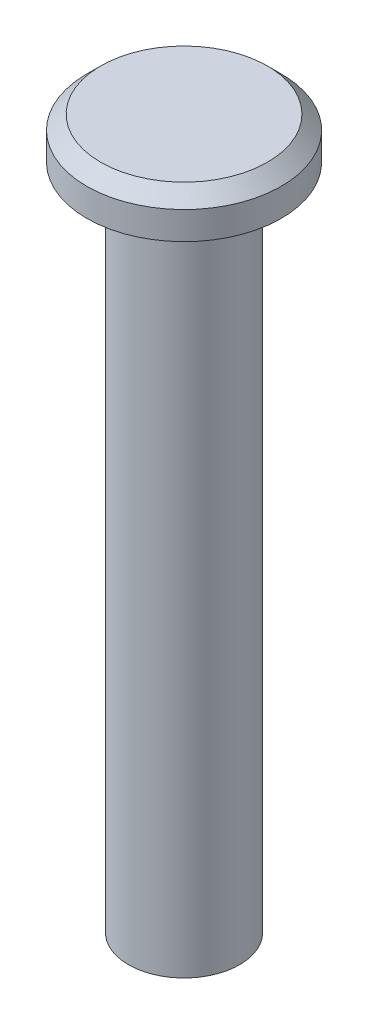
ISO-10303-21;
HEADER;
FILE_DESCRIPTION(('STEP AP214'),'2;1');
FILE_NAME('part.step','',(''),(''),'','','');
FILE_SCHEMA(('AUTOMOTIVE_DESIGN { 1 0 10303 214 1 1 1 1 }'));
ENDSEC;
DATA;
#1=APPLICATION_CONTEXT('core data for automotive mechanical design processes');
#2=APPLICATION_PROTOCOL_DEFINITION('international standard','automotive_design',2000,#1);
#3=PRODUCT_CONTEXT('',#1,'mechanical');
#4=PRODUCT('Part','Part','',(#3));
#5=PRODUCT_RELATED_PRODUCT_CATEGORY('part','',(#4));
#6=PRODUCT_DEFINITION_FORMATION('','',#4);
#7=PRODUCT_DEFINITION_CONTEXT('part definition',#1,'design');
#8=PRODUCT_DEFINITION('design','',#6,#7);
#9=PRODUCT_DEFINITION_SHAPE('','',#8);
#10=(LENGTH_UNIT() NAMED_UNIT(*) SI_UNIT(.MILLI.,.METRE.));
#11=(NAMED_UNIT(*) PLANE_ANGLE_UNIT() SI_UNIT($,.RADIAN.));
#12=(NAMED_UNIT(*) SI_UNIT($,.STERADIAN.) SOLID_ANGLE_UNIT());
#13=UNCERTAINTY_MEASURE_WITH_UNIT(LENGTH_MEASURE(1.E-05),#10,'distance_accuracy_value','');
#14=(GEOMETRIC_REPRESENTATION_CONTEXT(3) GLOBAL_UNCERTAINTY_ASSIGNED_CONTEXT((#13)) GLOBAL_UNIT_ASSIGNED_CONTEXT((#10,
#11,#12)) REPRESENTATION_CONTEXT('',''));
#15=CARTESIAN_POINT('',(0.,0.,0.));
#16=DIRECTION('',(0.,0.,1.));
#17=DIRECTION('',(1.,0.,0.));
#18=AXIS2_PLACEMENT_3D('',#15,#16,#17);
#19=CARTESIAN_POINT('',(0.,48.,0.));
#20=DIRECTION('',(0.,-1.,0.));
#21=DIRECTION('',(0.,0.,-1.));
#22=AXIS2_PLACEMENT_3D('',#19,#20,#21);
#23=CYLINDRICAL_SURFACE('',#22,4.);
#24=CARTESIAN_POINT('',(0.,48.,0.));
#25=DIRECTION('',(0.,1.,0.));
#26=DIRECTION('',(0.,0.,1.));
#27=AXIS2_PLACEMENT_3D('',#24,#25,#26);
#28=CIRCLE('',#27,4.);
#29=CARTESIAN_POINT('',(0.,48.,4.));
#30=VERTEX_POINT('',#29);
#31=EDGE_CURVE('E52',#30,#30,#28,.T.);
#32=ORIENTED_EDGE('',*,*,#31,.F.);
#33=EDGE_LOOP('',(#32));
#34=FACE_BOUND('',#33,.T.);
#35=CARTESIAN_POINT('',(0.,0.,0.));
#36=DIRECTION('',(0.,1.,0.));
#37=DIRECTION('',(0.,0.,1.));
#38=AXIS2_PLACEMENT_3D('',#35,#36,#37);
#39=CIRCLE('',#38,4.);
#40=CARTESIAN_POINT('',(0.,0.,4.));
#41=VERTEX_POINT('',#40);
#42=EDGE_CURVE('E60',#41,#41,#39,.T.);
#43=ORIENTED_EDGE('',*,*,#42,.T.);
#44=EDGE_LOOP('',(#43));
#45=FACE_BOUND('',#44,.T.);
#46=ADVANCED_FACE('F41',(#34,#45),#23,.T.);
#47=CARTESIAN_POINT('',(0.,0.,0.));
#48=DIRECTION('',(0.,1.,0.));
#49=DIRECTION('',(0.,0.,1.));
#50=AXIS2_PLACEMENT_3D('',#47,#48,#49);
#51=PLANE('',#50);
#52=ORIENTED_EDGE('',*,*,#42,.F.);
#53=EDGE_LOOP('',(#52));
#54=FACE_BOUND('',#53,.T.);
#55=ADVANCED_FACE('F83',(#54),#51,.F.);
#56=CARTESIAN_POINT('',(0.,51.,0.));
#57=DIRECTION('',(0.,-1.,0.));
#58=DIRECTION('',(0.,0.,-1.));
#59=AXIS2_PLACEMENT_3D('',#56,#57,#58);
#60=CYLINDRICAL_SURFACE('',#59,7.);
#61=CARTESIAN_POINT('',(0.,50.,0.));
#62=DIRECTION('',(0.,1.,0.));
#63=DIRECTION('',(0.,0.,1.));
#64=AXIS2_PLACEMENT_3D('',#61,#62,#63);
#65=CIRCLE('',#64,7.);
#66=CARTESIAN_POINT('',(0.,50.,7.));
#67=VERTEX_POINT('',#66);
#68=EDGE_CURVE('E10',#67,#67,#65,.F.);
#69=ORIENTED_EDGE('',*,*,#68,.T.);
#70=EDGE_LOOP('',(#69));
#71=FACE_BOUND('',#70,.T.);
#72=CARTESIAN_POINT('',(0.,48.,0.));
#73=DIRECTION('',(0.,1.,0.));
#74=DIRECTION('',(0.,0.,1.));
#75=AXIS2_PLACEMENT_3D('',#72,#73,#74);
#76=CIRCLE('',#75,7.);
#77=CARTESIAN_POINT('',(0.,48.,7.));
#78=VERTEX_POINT('',#77);
#79=EDGE_CURVE('E61',#78,#78,#76,.T.);
#80=ORIENTED_EDGE('',*,*,#79,.T.);
#81=EDGE_LOOP('',(#80));
#82=FACE_BOUND('',#81,.T.);
#83=ADVANCED_FACE('F66',(#71,#82),#60,.T.);
#84=CARTESIAN_POINT('',(0.,51.,0.));
#85=DIRECTION('',(0.,1.,0.));
#86=DIRECTION('',(0.,0.,1.));
#87=AXIS2_PLACEMENT_3D('',#84,#85,#86);
#88=PLANE('',#87);
#89=CARTESIAN_POINT('',(0.,51.,0.));
#90=DIRECTION('',(0.,1.,0.));
#91=DIRECTION('',(0.,0.,1.));
#92=AXIS2_PLACEMENT_3D('',#89,#90,#91);
#93=CIRCLE('',#92,6.);
#94=CARTESIAN_POINT('',(0.,51.,6.));
#95=VERTEX_POINT('',#94);
#96=EDGE_CURVE('E47',#95,#95,#93,.T.);
#97=ORIENTED_EDGE('',*,*,#96,.T.);
#98=EDGE_LOOP('',(#97));
#99=FACE_BOUND('',#98,.T.);
#100=ADVANCED_FACE('F69',(#99),#88,.T.);
#101=CARTESIAN_POINT('',(0.,48.,0.));
#102=DIRECTION('',(0.,1.,0.));
#103=DIRECTION('',(0.,0.,1.));
#104=AXIS2_PLACEMENT_3D('',#101,#102,#103);
#105=PLANE('',#104);
#106=ORIENTED_EDGE('',*,*,#31,.T.);
#107=EDGE_LOOP('',(#106));
#108=FACE_BOUND('',#107,.T.);
#109=ORIENTED_EDGE('',*,*,#79,.F.);
#110=EDGE_LOOP('',(#109));
#111=FACE_BOUND('',#110,.T.);
#112=ADVANCED_FACE('F68',(#108,#111),#105,.F.);
#113=CARTESIAN_POINT('',(0.,51.,0.));
#114=DIRECTION('',(0.,-1.,0.));
#115=DIRECTION('',(0.,0.,-1.));
#116=AXIS2_PLACEMENT_3D('',#113,#114,#115);
#117=CONICAL_SURFACE('',#116,6.,0.785398163397445);
#118=ORIENTED_EDGE('',*,*,#68,.F.);
#119=EDGE_LOOP('',(#118));
#120=FACE_BOUND('',#119,.T.);
#121=ORIENTED_EDGE('',*,*,#96,.F.);
#122=EDGE_LOOP('',(#121));
#123=FACE_BOUND('',#122,.T.);
#124=ADVANCED_FACE('F42',(#120,#123),#117,.T.);
#125=CLOSED_SHELL('',(#46,#55,#83,#100,#112,#124));
#126=MANIFOLD_SOLID_BREP('B2',#125);
#127=ADVANCED_BREP_SHAPE_REPRESENTATION('',(#18,#126),#14);
#128=SHAPE_DEFINITION_REPRESENTATION(#9,#127);
ENDSEC;
END-ISO-10303-21;
